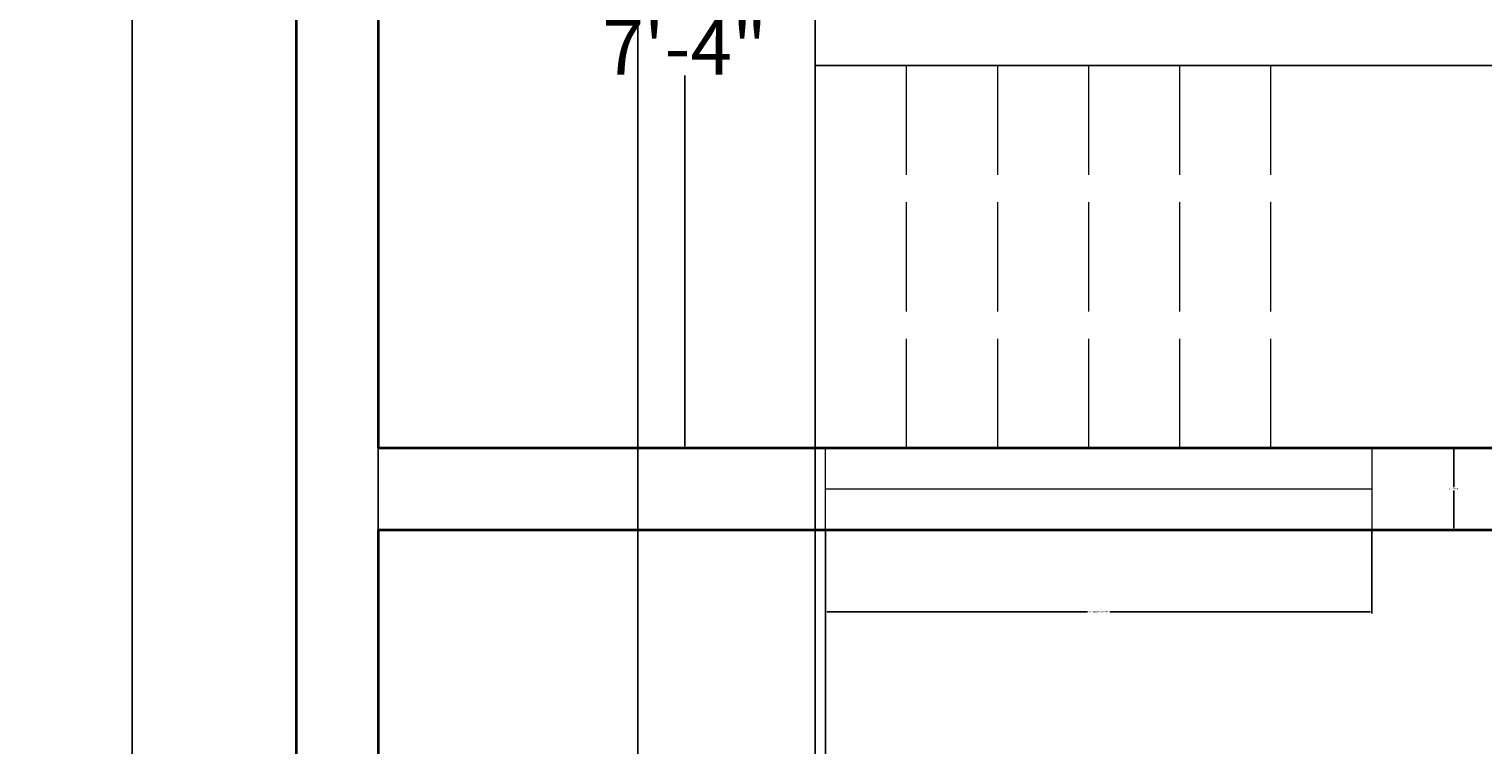
# Model space of a CAD drawing. Units: inches. Extents: x -10 to 502, y -868 to 56.
# Tile 6 of 14: x 6 to 165, y -573 to -495. Entities that reach past the tile are written whole.
import ezdxf

# ---------------------------------------------------------------- set-up
doc = ezdxf.new("R2010")
doc.units = ezdxf.units.IN
doc.header["$MEASUREMENT"] = 0
doc.linetypes.add('ACAD_ISO02W100', pattern=[15, 12, -3])
for name, color, linetype, lineweight in [('A-ANNO-DIMS', 2, 'Continuous', 18), ('A-FLOR-STRS', 7, 'Continuous', 25), ('A-FLOR-STRS-HIDN', 7, 'ACAD_ISO02W100', 18), ('A-GLAZ', 162, 'Continuous', 18), ('A-WALL', 7, 'Continuous', 35), ('L-WALL', 7, 'Continuous', 35)]:
    doc.layers.add(name, color=color, linetype=linetype, lineweight=lineweight)
doc.styles.get("Standard").update_dxf_attribs({"font": 'arial.ttf'})
doc.dimstyles.get("Standard").update_dxf_attribs({"dimtxt": 0.18, "dimasz": 0.18, "dimexe": 0.18, "dimexo": 0.0625, "dimgap": 0.09, "dimtad": 0, "dimtih": 1, "dimtoh": 1, "dimdec": 0, "dimzin": 0, "dimdsep": 46, "dimlunit": 3, "dimtxsty": 'Standard', "dimcen": 0.09, "dimadec": 0, "dimazin": 0, "dimtfac": 1, "dimtdec": 0, "dimtofl": 0, "dimtmove": 0, "dimatfit": 3, "dimfxl": 1, "dimtolj": 1, "dimtzin": 0, "dimarcsym": 0})

# ---------------------------------------------------------------- blocks, each defined once
blk = doc.blocks.new('*D2')
at = {"layer": 'A-ANNO-DIMS', "color": 0, "lineweight": -2, "transparency": 16777216}
for p, q in [((34.89, 12.15), (16.75, 12.15)), ((16.93, 11.97), (16.93, -376.2)), ((16.93, -770.67), (16.93, -382.51)), ((34.89, -770.85), (16.75, -770.85))]:
    blk.add_line(p, q, dxfattribs=at)
at = {"layer": 'A-ANNO-DIMS', "color": 0, "transparency": 16777216}
for points in [[(16.9, 11.97), (16.96, 11.97), (16.93, 12.15)], [(16.9, -770.67), (16.96, -770.67), (16.93, -770.85)]]:
    blk.add_solid(points, dxfattribs=at)
at = {"layer": 'Defpoints', "color": 0, "transparency": 16777216}
for p in [(34.95, 12.15), (16.93, -770.85), (34.95, -770.85)]:
    blk.add_point(p, dxfattribs=at)
at = {"layer": 'A-ANNO-DIMS', "color": 0, "transparency": 16777216, "insert": (16.93, -379.35), "char_height": 6, "attachment_point": 5}
blk.add_mtext('\\A1;65\'-3"', dxfattribs=at)
blk = doc.blocks.new('*D6')
at = {"layer": 'A-ANNO-DIMS', "color": 0, "lineweight": -2, "transparency": 16777216}
for p, q in [((76.89, -452.85), (77.81, -452.85)), ((77.63, -453.03), (77.63, -493.76)), ((77.63, -540.67), (77.63, -499.94)), ((76.89, -540.85), (77.81, -540.85))]:
    blk.add_line(p, q, dxfattribs=at)
at = {"layer": 'A-ANNO-DIMS', "color": 0, "transparency": 16777216}
for points in [[(77.6, -453.03), (77.66, -453.03), (77.63, -452.85)], [(77.6, -540.67), (77.66, -540.67), (77.63, -540.85)]]:
    blk.add_solid(points, dxfattribs=at)
at = {"layer": 'Defpoints', "color": 0, "transparency": 16777216}
for p in [(76.83, -452.85), (76.83, -540.85), (77.63, -540.85)]:
    blk.add_point(p, dxfattribs=at)
at = {"layer": 'A-ANNO-DIMS', "color": 0, "transparency": 16777216, "insert": (77.63, -496.85), "char_height": 6, "attachment_point": 5}
blk.add_mtext('\\A1;7\'-4"', dxfattribs=at)
blk = doc.blocks.new('WIN-60IN')
for p, q in [((0, 9), (60, 9)), ((0, 0), (0, 9)), ((60, 9), (60, 0)), ((0, 4.5), (60, 4.5)), ((60, 0), (0, 0))]:
    blk.add_line(p, q)
blk = doc.blocks.new('*D19')
at = {"layer": 'A-ANNO-DIMS', "color": 0, "lineweight": -2, "transparency": 16777216}
for p, q in [((93.07, -549.92), (93.07, -559.03)), ((153.07, -549.92), (153.07, -559.03)), ((93.25, -558.85), (121.84, -558.85)), ((152.89, -558.85), (124.3, -558.85))]:
    blk.add_line(p, q, dxfattribs=at)
at = {"layer": 'A-ANNO-DIMS', "color": 0, "transparency": 16777216}
for points in [[(93.25, -558.82), (93.25, -558.88), (93.07, -558.85)], [(152.89, -558.82), (152.89, -558.88), (153.07, -558.85)]]:
    blk.add_solid(points, dxfattribs=at)
at = {"layer": 'Defpoints', "color": 0, "transparency": 16777216}
for p in [(93.07, -549.85), (153.07, -549.85), (153.07, -558.85)]:
    blk.add_point(p, dxfattribs=at)
at = {"layer": 'A-ANNO-DIMS', "color": 0, "transparency": 16777216, "insert": (123.07, -558.85), "char_height": 0.18, "attachment_point": 5}
blk.add_mtext('\\A1;WINDOW 5\'-0" TYP.', dxfattribs=at)
blk = doc.blocks.new('*D20')
at = {"layer": 'A-ANNO-DIMS', "color": 0, "lineweight": -2, "transparency": 16777216}
for p, q in [((153.14, -540.85), (162.25, -540.85)), ((162.07, -541.03), (162.07, -545.17)), ((162.07, -549.67), (162.07, -545.53)), ((153.14, -549.85), (162.25, -549.85))]:
    blk.add_line(p, q, dxfattribs=at)
at = {"layer": 'A-ANNO-DIMS', "color": 0, "transparency": 16777216}
for points in [[(162.04, -541.03), (162.1, -541.03), (162.07, -540.85)], [(162.04, -549.67), (162.1, -549.67), (162.07, -549.85)]]:
    blk.add_solid(points, dxfattribs=at)
at = {"layer": 'Defpoints', "color": 0, "transparency": 16777216}
for p in [(153.07, -540.85), (162.07, -540.85), (153.07, -549.85)]:
    blk.add_point(p, dxfattribs=at)
at = {"layer": 'A-ANNO-DIMS', "color": 0, "transparency": 16777216, "insert": (162.07, -545.35), "char_height": 0.18, "attachment_point": 5}
blk.add_mtext('\\A1;0\'-9" TYP.', dxfattribs=at)
blk = doc.blocks.new('*D47')
at = {"layer": 'A-ANNO-DIMS', "color": 0, "lineweight": -2, "transparency": 16777216}
for p, q in [((91.95, -494.92), (91.95, -846.58)), ((201.95, -494.92), (201.95, -846.58)), ((92.13, -846.4), (146.62, -846.4)), ((201.77, -846.4), (147.28, -846.4))]:
    blk.add_line(p, q, dxfattribs=at)
at = {"layer": 'A-ANNO-DIMS', "color": 0, "transparency": 16777216}
for points in [[(92.13, -846.37), (92.13, -846.43), (91.95, -846.4)], [(201.77, -846.37), (201.77, -846.43), (201.95, -846.4)]]:
    blk.add_solid(points, dxfattribs=at)
at = {"layer": 'Defpoints', "color": 0, "transparency": 16777216}
for p in [(91.95, -494.85), (201.95, -494.85), (201.95, -846.4)]:
    blk.add_point(p, dxfattribs=at)
at = {"layer": 'A-ANNO-DIMS', "color": 0, "transparency": 16777216, "insert": (146.95, -846.4), "char_height": 0.18, "attachment_point": 5}
blk.add_mtext('\\A1;9\'-2"', dxfattribs=at)
blk = doc.blocks.new('*D48')
at = {"layer": 'A-ANNO-DIMS', "color": 0, "lineweight": -2, "transparency": 16777216}
for p, q in [((43.95, -332.92), (43.95, -846.58)), ((72.45, -332.92), (72.45, -846.58)), ((44.13, -846.4), (57.66, -846.4)), ((72.27, -846.4), (58.74, -846.4))]:
    blk.add_line(p, q, dxfattribs=at)
at = {"layer": 'A-ANNO-DIMS', "color": 0, "transparency": 16777216}
for points in [[(44.13, -846.37), (44.13, -846.43), (43.95, -846.4)], [(72.27, -846.37), (72.27, -846.43), (72.45, -846.4)]]:
    blk.add_solid(points, dxfattribs=at)
at = {"layer": 'Defpoints', "color": 0, "transparency": 16777216}
for p in [(43.95, -332.85), (72.45, -332.85), (72.45, -846.4)]:
    blk.add_point(p, dxfattribs=at)
at = {"layer": 'A-ANNO-DIMS', "color": 0, "transparency": 16777216, "insert": (58.2, -846.4), "char_height": 0.18, "attachment_point": 5}
blk.add_mtext('\\A1;2\'-4 1/2"', dxfattribs=at)
blk = doc.blocks.new('*D56')
at = {"layer": 'A-ANNO-DIMS', "color": 0, "lineweight": -2, "transparency": 16777216}
for p, q in [((43.95, -549.92), (43.95, -846.58)), ((93.07, -549.92), (93.07, -846.58)), ((44.13, -846.4), (68.18, -846.4)), ((92.89, -846.4), (68.84, -846.4))]:
    blk.add_line(p, q, dxfattribs=at)
at = {"layer": 'A-ANNO-DIMS', "color": 0, "transparency": 16777216}
for points in [[(44.13, -846.37), (44.13, -846.43), (43.95, -846.4)], [(92.89, -846.37), (92.89, -846.43), (93.07, -846.4)]]:
    blk.add_solid(points, dxfattribs=at)
at = {"layer": 'Defpoints', "color": 0, "transparency": 16777216}
for p in [(43.95, -549.85), (93.07, -549.85), (43.95, -846.4)]:
    blk.add_point(p, dxfattribs=at)
at = {"layer": 'A-ANNO-DIMS', "color": 0, "transparency": 16777216, "insert": (68.51, -846.4), "char_height": 0.18, "attachment_point": 5}
blk.add_mtext('\\A1;4\'-1"', dxfattribs=at)

msp = doc.modelspace()

# ---------------------------------------------------------------- linework, layer by layer
at = {"layer": 'A-FLOR-STRS'}
for p, q in [((91.95, -452.85), (91.95, -498.85)), ((91.95, -498.85), (201.95, -498.85))]:
    msp.add_line(p, q, dxfattribs=at)
at = {"layer": 'A-FLOR-STRS-HIDN'}
for p, q in [((91.95, -498.85), (91.95, -540.85)), ((101.95, -498.85), (101.95, -540.85)), ((111.95, -498.85), (111.95, -540.85)), ((121.95, -498.85), (121.95, -540.85)), ((131.95, -498.85), (131.95, -540.85)), ((141.95, -498.85), (141.95, -540.85))]:
    msp.add_line(p, q, dxfattribs=at)
at = {"layer": 'A-WALL'}
for p, q in [((34.95, 12.15), (34.95, -770.85)), ((43.95, -452.85), (43.95, -540.85)), ((43.95, -540.85), (211.95, -540.85)), ((43.95, -549.85), (271.95, -549.85))]:
    msp.add_line(p, q, dxfattribs=at)
at = {"layer": 'L-WALL'}
msp.add_line((43.95, -549.85), (43.95, -770.85), dxfattribs=at)

# ---------------------------------------------------------------- block references
at = {"layer": 'A-GLAZ'}
msp.add_blockref('WIN-60IN', (93.07, -549.85), dxfattribs=at)

# ---------------------------------------------------------------- dimensions: what is measured, and where the dimension line sits
at = {"layer": 'A-ANNO-DIMS'}
for base, p1, p2, picture, middle in [((16.93, -770.85), (34.95, 12.15), (34.95, -770.85), '*D2', (16.93, -379.35)), ((77.63, -540.85), (76.83, -452.85), (76.83, -540.85), '*D6', (77.63, -496.85))]:
    dim = msp.add_linear_dim(base=base, p1=p1, p2=p2, angle=90, dimstyle='Standard', override={"dimtxt": 6, "dimclrd": 0, "dimclre": 0, "dimclrt": 0}, dxfattribs=at)
    dim.commit()
    dim.dimension.update_dxf_attribs({"geometry": picture, "text_midpoint": middle})
for base, p1, p2, picture, middle in [((72.45, -846.4), (43.95, -332.85), (72.45, -332.85), '*D48', (58.2, -846.4)), ((201.95, -846.4), (91.95, -494.85), (201.95, -494.85), '*D47', (146.95, -846.4)), ((43.95, -846.4), (93.07, -549.85), (43.95, -549.85), '*D56', (68.51, -846.4))]:
    dim = msp.add_linear_dim(base=base, p1=p1, p2=p2, dimstyle='Standard', override={"dimdec": 1, "dimlfac": 1, "dimrnd": 0, "dimzin": 1, "dimdsep": 46, "dimlunit": 4, "dimfrac": 2}, dxfattribs=at)
    dim.commit()
    dim.dimension.update_dxf_attribs({"geometry": picture, "text_midpoint": middle})
dim = msp.add_linear_dim(base=(162.07, -540.85), p1=(153.07, -549.85), p2=(153.07, -540.85), angle=90, text='<> TYP.', dimstyle='Standard', override={"dimdec": 1, "dimlfac": 1, "dimrnd": 0, "dimzin": 1, "dimdsep": 46, "dimlunit": 4, "dimfrac": 2}, dxfattribs=at)
dim.commit()
dim.dimension.update_dxf_attribs({"geometry": '*D20', "text_midpoint": (162.07, -545.35)})
dim = msp.add_linear_dim(base=(153.07, -558.85), p1=(93.07, -549.85), p2=(153.07, -549.85), text='WINDOW <> TYP.', dimstyle='Standard', override={"dimdec": 1, "dimlfac": 1, "dimrnd": 0, "dimzin": 1, "dimdsep": 46, "dimlunit": 4, "dimfrac": 2}, dxfattribs=at)
dim.commit()
dim.dimension.update_dxf_attribs({"geometry": '*D19', "text_midpoint": (123.07, -558.85)})

doc.saveas('drawing.dxf')
